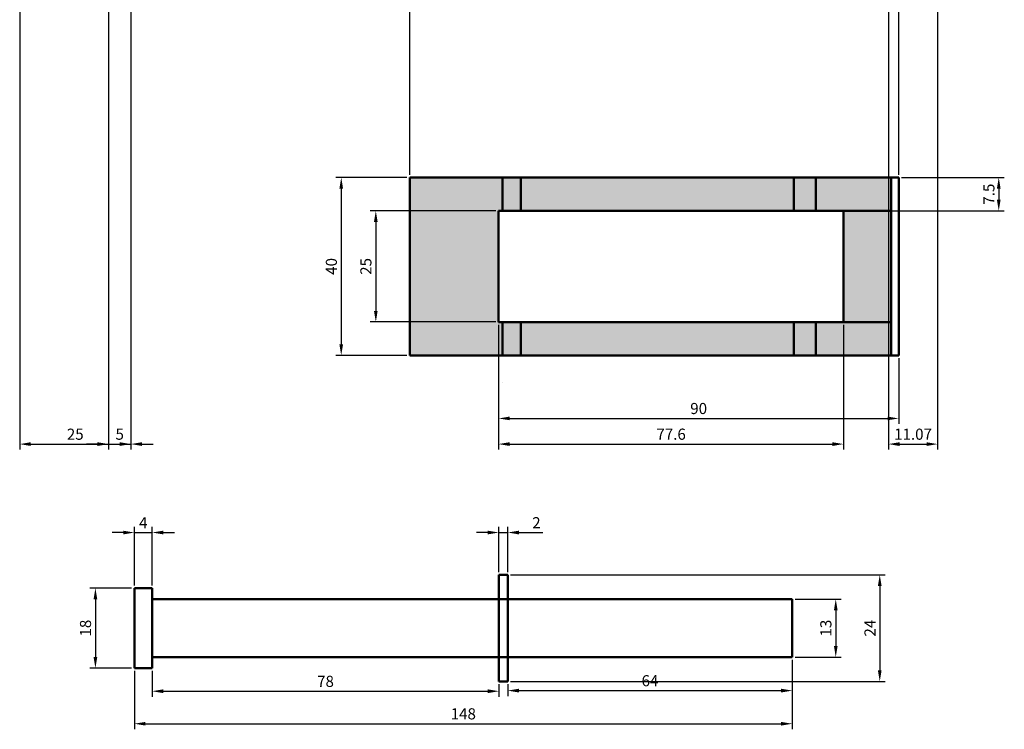
# Model space of a CAD drawing. Units: millimetres. Extents: x 2180 to 2428, y 1025 to 1371.
# Tile 1 of 3: x 2201 to 2422, y 1025 to 1185. Entities that reach past the tile are written whole.
import ezdxf

# ---------------------------------------------------------------- set-up
doc = ezdxf.new("R2010")
doc.units = ezdxf.units.MM
for name, color, linetype, lineweight in [('M-CONS', 8, 'Continuous', 13), ('M-DIMS', 2, 'Continuous', 25), ('M-HATC', 252, 'Continuous', 18), ('M-OUTL', 7, 'Continuous', 50)]:
    doc.layers.add(name, color=color, linetype=linetype, lineweight=lineweight)
doc.styles.get("Standard").update_dxf_attribs({"font": 'arial.ttf'})
doc.dimstyles.new('ISO-25', dxfattribs={"dimtxt": 2.5, "dimasz": 2.5, "dimexe": 1.25, "dimexo": 0.625, "dimtad": 1, "dimtxsty": 'Standard', "dimcen": 2.5, "dimadec": 0, "dimazin": 0, "dimtfac": 1, "dimtmove": 0, "dimatfit": 3, "dimfxl": 1, "dimarcsym": 0})

# ---------------------------------------------------------------- blocks, each defined once
blk = doc.blocks.new('*D22')
at = {"layer": 'Defpoints', "color": 0, "transparency": 16777216}
for p in [(2308.57, 1117), (2398.57, 1109.5), (2398.57, 1095.31)]:
    blk.add_point(p, dxfattribs=at)
at = {"layer": 'M-DIMS', "color": 0, "lineweight": -2, "transparency": 16777216}
for p, q in [((2308.57, 1116.37), (2308.57, 1094.06)), ((2398.57, 1108.87), (2398.57, 1094.06)), ((2311.07, 1095.31), (2396.07, 1095.31))]:
    blk.add_line(p, q, dxfattribs=at)
at = {"layer": 'M-DIMS', "color": 0, "transparency": 16777216}
for points in [[(2311.07, 1095.73), (2311.07, 1094.9), (2308.57, 1095.31)], [(2396.07, 1095.73), (2396.07, 1094.9), (2398.57, 1095.31)]]:
    blk.add_solid(points, dxfattribs=at)
at = {"layer": 'M-DIMS', "color": 0, "transparency": 16777216, "insert": (2353.57, 1097.22), "char_height": 2.5, "attachment_point": 5}
blk.add_mtext('90', dxfattribs=at)
blk = doc.blocks.new('*D23')
at = {"layer": 'Defpoints', "color": 0, "transparency": 16777216}
for p in [(2308.57, 1142), (2280.94, 1117), (2308.57, 1117)]:
    blk.add_point(p, dxfattribs=at)
at = {"layer": 'M-DIMS', "color": 0, "lineweight": -2, "transparency": 16777216}
for p, q in [((2307.95, 1142), (2279.69, 1142)), ((2280.94, 1139.5), (2280.94, 1119.5)), ((2307.95, 1117), (2279.69, 1117))]:
    blk.add_line(p, q, dxfattribs=at)
at = {"layer": 'M-DIMS', "color": 0, "transparency": 16777216}
for points in [[(2280.52, 1139.5), (2281.35, 1139.5), (2280.94, 1142)], [(2280.52, 1119.5), (2281.35, 1119.5), (2280.94, 1117)]]:
    blk.add_solid(points, dxfattribs=at)
at = {"layer": 'M-DIMS', "color": 0, "transparency": 16777216, "insert": (2279.03, 1129.5), "char_height": 2.5, "attachment_point": 5, "rotation": 90}
blk.add_mtext('25', dxfattribs=at)
blk = doc.blocks.new('*D24')
at = {"layer": 'Defpoints', "color": 0, "transparency": 16777216}
for p in [(2288.57, 1149.5), (2273.16, 1109.5), (2288.57, 1109.5)]:
    blk.add_point(p, dxfattribs=at)
at = {"layer": 'M-DIMS', "color": 0, "lineweight": -2, "transparency": 16777216}
for p, q in [((2287.95, 1149.5), (2271.91, 1149.5)), ((2273.16, 1147), (2273.16, 1112)), ((2287.95, 1109.5), (2271.91, 1109.5))]:
    blk.add_line(p, q, dxfattribs=at)
at = {"layer": 'M-DIMS', "color": 0, "transparency": 16777216}
for points in [[(2272.74, 1147), (2273.57, 1147), (2273.16, 1149.5)], [(2272.74, 1112), (2273.57, 1112), (2273.16, 1109.5)]]:
    blk.add_solid(points, dxfattribs=at)
at = {"layer": 'M-DIMS', "color": 0, "transparency": 16777216, "insert": (2271.26, 1129.5), "char_height": 2.5, "attachment_point": 5, "rotation": 90}
blk.add_mtext('40', dxfattribs=at)
blk = doc.blocks.new('*D25')
at = {"layer": 'Defpoints', "color": 0, "transparency": 16777216}
for p in [(2230.62, 1039.15), (2308.62, 1036.15), (2308.62, 1033.96)]:
    blk.add_point(p, dxfattribs=at)
at = {"layer": 'M-DIMS', "color": 0, "lineweight": -2, "transparency": 16777216}
for p, q in [((2230.62, 1038.52), (2230.62, 1032.71)), ((2308.62, 1035.52), (2308.62, 1032.71)), ((2233.12, 1033.96), (2306.12, 1033.96))]:
    blk.add_line(p, q, dxfattribs=at)
at = {"layer": 'M-DIMS', "color": 0, "transparency": 16777216}
for points in [[(2233.12, 1034.38), (2233.12, 1033.54), (2230.62, 1033.96)], [(2306.12, 1034.38), (2306.12, 1033.54), (2308.62, 1033.96)]]:
    blk.add_solid(points, dxfattribs=at)
at = {"layer": 'M-DIMS', "color": 0, "transparency": 16777216, "insert": (2269.62, 1035.86), "char_height": 2.5, "attachment_point": 5}
blk.add_mtext('78', dxfattribs=at)
blk = doc.blocks.new('*D26')
at = {"layer": 'Defpoints', "color": 0, "transparency": 16777216}
for p in [(2374.62, 1041.65), (2310.62, 1036.15), (2374.62, 1034.1)]:
    blk.add_point(p, dxfattribs=at)
at = {"layer": 'M-DIMS', "color": 0, "lineweight": -2, "transparency": 16777216}
for p, q in [((2374.62, 1041.02), (2374.62, 1032.85)), ((2310.62, 1035.52), (2310.62, 1032.85)), ((2313.12, 1034.1), (2372.12, 1034.1))]:
    blk.add_line(p, q, dxfattribs=at)
at = {"layer": 'M-DIMS', "color": 0, "transparency": 16777216}
for points in [[(2313.12, 1034.52), (2313.12, 1033.68), (2310.62, 1034.1)], [(2372.12, 1034.52), (2372.12, 1033.68), (2374.62, 1034.1)]]:
    blk.add_solid(points, dxfattribs=at)
at = {"layer": 'M-DIMS', "color": 0, "transparency": 16777216, "insert": (2342.62, 1036), "char_height": 2.5, "attachment_point": 5}
blk.add_mtext('64', dxfattribs=at)
blk = doc.blocks.new('*D27')
at = {"layer": 'Defpoints', "color": 0, "transparency": 16777216}
for p in [(2226.62, 1057.15), (2217.85, 1039.15), (2226.62, 1039.15)]:
    blk.add_point(p, dxfattribs=at)
at = {"layer": 'M-DIMS', "color": 0, "lineweight": -2, "transparency": 16777216}
for p, q in [((2226, 1057.15), (2216.6, 1057.15)), ((2217.85, 1054.65), (2217.85, 1041.65)), ((2226, 1039.15), (2216.6, 1039.15))]:
    blk.add_line(p, q, dxfattribs=at)
at = {"layer": 'M-DIMS', "color": 0, "transparency": 16777216}
for points in [[(2217.44, 1054.65), (2218.27, 1054.65), (2217.85, 1057.15)], [(2217.44, 1041.65), (2218.27, 1041.65), (2217.85, 1039.15)]]:
    blk.add_solid(points, dxfattribs=at)
at = {"layer": 'M-DIMS', "color": 0, "transparency": 16777216, "insert": (2215.95, 1048.15), "char_height": 2.5, "attachment_point": 5, "rotation": 90}
blk.add_mtext('18', dxfattribs=at)
blk = doc.blocks.new('*D28')
at = {"layer": 'Defpoints', "color": 0, "transparency": 16777216}
for p in [(2310.62, 1060.15), (2310.62, 1036.15), (2394.31, 1036.15)]:
    blk.add_point(p, dxfattribs=at)
at = {"layer": 'M-DIMS', "color": 0, "lineweight": -2, "transparency": 16777216}
for p, q in [((2311.25, 1060.15), (2395.56, 1060.15)), ((2394.31, 1057.65), (2394.31, 1038.65)), ((2311.25, 1036.15), (2395.56, 1036.15))]:
    blk.add_line(p, q, dxfattribs=at)
at = {"layer": 'M-DIMS', "color": 0, "transparency": 16777216}
for points in [[(2393.89, 1057.65), (2394.72, 1057.65), (2394.31, 1060.15)], [(2393.89, 1038.65), (2394.72, 1038.65), (2394.31, 1036.15)]]:
    blk.add_solid(points, dxfattribs=at)
at = {"layer": 'M-DIMS', "color": 0, "transparency": 16777216, "insert": (2392.43, 1048.15), "char_height": 2.5, "attachment_point": 5, "rotation": 90}
blk.add_mtext('24', dxfattribs=at)
blk = doc.blocks.new('*D29')
at = {"layer": 'Defpoints', "color": 0, "transparency": 16777216}
for p in [(2374.62, 1054.65), (2374.62, 1041.65), (2384.41, 1041.65)]:
    blk.add_point(p, dxfattribs=at)
at = {"layer": 'M-DIMS', "color": 0, "lineweight": -2, "transparency": 16777216}
for p, q in [((2375.25, 1054.65), (2385.66, 1054.65)), ((2384.41, 1052.15), (2384.41, 1044.15)), ((2375.25, 1041.65), (2385.66, 1041.65))]:
    blk.add_line(p, q, dxfattribs=at)
at = {"layer": 'M-DIMS', "color": 0, "transparency": 16777216}
for points in [[(2384, 1052.15), (2384.83, 1052.15), (2384.41, 1054.65)], [(2384, 1044.15), (2384.83, 1044.15), (2384.41, 1041.65)]]:
    blk.add_solid(points, dxfattribs=at)
at = {"layer": 'M-DIMS', "color": 0, "transparency": 16777216, "insert": (2382.51, 1048.15), "char_height": 2.5, "attachment_point": 5, "rotation": 90}
blk.add_mtext('13', dxfattribs=at)
blk = doc.blocks.new('*D30')
at = {"layer": 'Defpoints', "color": 0, "transparency": 16777216}
for p in [(2200.82, 1194.18), (2225.82, 1194.18), (2225.82, 1089.54)]:
    blk.add_point(p, dxfattribs=at)
at = {"layer": 'M-DIMS', "color": 0, "lineweight": -2, "transparency": 16777216}
for p, q in [((2200.82, 1193.55), (2200.82, 1088.29)), ((2225.82, 1193.55), (2225.82, 1088.29)), ((2203.32, 1089.54), (2223.32, 1089.54))]:
    blk.add_line(p, q, dxfattribs=at)
at = {"layer": 'M-DIMS', "color": 0, "transparency": 16777216}
for points in [[(2203.32, 1089.96), (2203.32, 1089.12), (2200.82, 1089.54)], [(2223.32, 1089.96), (2223.32, 1089.12), (2225.82, 1089.54)]]:
    blk.add_solid(points, dxfattribs=at)
at = {"layer": 'M-DIMS', "color": 0, "transparency": 16777216, "insert": (2213.32, 1091.44), "char_height": 2.5, "attachment_point": 5}
blk.add_mtext('25', dxfattribs=at)
blk = doc.blocks.new('*D34')
at = {"layer": 'Defpoints', "color": 0, "transparency": 16777216}
for p in [(2220.82, 1234.18), (2225.82, 1234.18), (2225.82, 1089.54)]:
    blk.add_point(p, dxfattribs=at)
at = {"layer": 'M-DIMS', "color": 0, "lineweight": -2, "transparency": 16777216}
for p, q in [((2220.82, 1233.55), (2220.82, 1088.29)), ((2225.82, 1233.55), (2225.82, 1088.29)), ((2218.32, 1089.54), (2215.82, 1089.54)), ((2220.82, 1089.54), (2225.82, 1089.54)), ((2228.32, 1089.54), (2230.82, 1089.54))]:
    blk.add_line(p, q, dxfattribs=at)
at = {"layer": 'M-DIMS', "color": 0, "transparency": 16777216}
for points in [[(2218.32, 1089.96), (2218.32, 1089.12), (2220.82, 1089.54)], [(2228.32, 1089.96), (2228.32, 1089.12), (2225.82, 1089.54)]]:
    blk.add_solid(points, dxfattribs=at)
at = {"layer": 'M-DIMS', "color": 0, "transparency": 16777216, "insert": (2223.32, 1091.44), "char_height": 2.5, "attachment_point": 5}
blk.add_mtext('5', dxfattribs=at)
blk = doc.blocks.new('*D37')
at = {"layer": 'Defpoints', "color": 0, "transparency": 16777216}
for p in [(2396.26, 1228.33), (2407.33, 1228.24), (2407.33, 1089.54)]:
    blk.add_point(p, dxfattribs=at)
at = {"layer": 'M-DIMS', "color": 0, "lineweight": -2, "transparency": 16777216}
for p, q in [((2396.26, 1227.71), (2396.26, 1088.29)), ((2407.33, 1227.61), (2407.33, 1088.29)), ((2398.76, 1089.54), (2404.83, 1089.54))]:
    blk.add_line(p, q, dxfattribs=at)
at = {"layer": 'M-DIMS', "color": 0, "transparency": 16777216}
for points in [[(2398.76, 1089.96), (2398.76, 1089.12), (2396.26, 1089.54)], [(2404.83, 1089.96), (2404.83, 1089.12), (2407.33, 1089.54)]]:
    blk.add_solid(points, dxfattribs=at)
at = {"layer": 'M-DIMS', "color": 0, "transparency": 16777216, "insert": (2401.8, 1091.44), "char_height": 2.5, "attachment_point": 5}
blk.add_mtext('11.07', dxfattribs=at)
blk = doc.blocks.new('*D41')
at = {"layer": 'Defpoints', "color": 0, "transparency": 16777216}
for p in [(2398.57, 1367.93), (2288.57, 1149.5), (2398.57, 1149.5)]:
    blk.add_point(p, dxfattribs=at)
at = {"layer": 'M-DIMS', "color": 0, "lineweight": -2, "transparency": 16777216}
for p, q in [((2288.57, 1150.12), (2288.57, 1369.18)), ((2398.57, 1150.12), (2398.57, 1369.18)), ((2291.07, 1367.93), (2396.07, 1367.93))]:
    blk.add_line(p, q, dxfattribs=at)
at = {"layer": 'M-DIMS', "color": 0, "transparency": 16777216}
for points in [[(2291.07, 1368.35), (2291.07, 1367.51), (2288.57, 1367.93)], [(2396.07, 1368.35), (2396.07, 1367.51), (2398.57, 1367.93)]]:
    blk.add_solid(points, dxfattribs=at)
at = {"layer": 'M-DIMS', "color": 0, "transparency": 16777216, "insert": (2343.57, 1369.83), "char_height": 2.5, "attachment_point": 5}
blk.add_mtext('110', dxfattribs=at)
blk = doc.blocks.new('*D42')
at = {"layer": 'Defpoints', "color": 0, "transparency": 16777216}
for p in [(2308.57, 1117), (2386.17, 1117), (2386.17, 1089.54)]:
    blk.add_point(p, dxfattribs=at)
at = {"layer": 'M-DIMS', "color": 0, "lineweight": -2, "transparency": 16777216}
for p, q in [((2308.57, 1116.37), (2308.57, 1088.29)), ((2386.17, 1116.37), (2386.17, 1088.29)), ((2311.07, 1089.54), (2383.67, 1089.54))]:
    blk.add_line(p, q, dxfattribs=at)
at = {"layer": 'M-DIMS', "color": 0, "transparency": 16777216}
for points in [[(2311.07, 1089.96), (2311.07, 1089.12), (2308.57, 1089.54)], [(2383.67, 1089.96), (2383.67, 1089.12), (2386.17, 1089.54)]]:
    blk.add_solid(points, dxfattribs=at)
at = {"layer": 'M-DIMS', "color": 0, "transparency": 16777216, "insert": (2347.37, 1091.44), "char_height": 2.5, "attachment_point": 5}
blk.add_mtext('77.6', dxfattribs=at)
blk = doc.blocks.new('*D43')
at = {"layer": 'Defpoints', "color": 0, "transparency": 16777216}
for p in [(2398.57, 1149.5), (2386.17, 1142), (2421.08, 1142)]:
    blk.add_point(p, dxfattribs=at)
at = {"layer": 'M-DIMS', "color": 0, "lineweight": -2, "transparency": 16777216}
for p, q in [((2399.2, 1149.5), (2422.33, 1149.5)), ((2421.08, 1147), (2421.08, 1144.5)), ((2386.8, 1142), (2422.33, 1142))]:
    blk.add_line(p, q, dxfattribs=at)
at = {"layer": 'M-DIMS', "color": 0, "transparency": 16777216}
for points in [[(2420.67, 1147), (2421.5, 1147), (2421.08, 1149.5)], [(2420.67, 1144.5), (2421.5, 1144.5), (2421.08, 1142)]]:
    blk.add_solid(points, dxfattribs=at)
at = {"layer": 'M-DIMS', "color": 0, "transparency": 16777216, "insert": (2419.19, 1145.75), "char_height": 2.5, "attachment_point": 5, "rotation": 90}
blk.add_mtext('7.5', dxfattribs=at)
blk = doc.blocks.new('*D44')
at = {"layer": 'Defpoints', "color": 0, "transparency": 16777216}
for p in [(2374.62, 1041.65), (2226.62, 1039.15), (2374.62, 1026.65)]:
    blk.add_point(p, dxfattribs=at)
at = {"layer": 'M-DIMS', "color": 0, "lineweight": -2, "transparency": 16777216}
for p, q in [((2374.62, 1041.02), (2374.62, 1025.4)), ((2226.62, 1038.52), (2226.62, 1025.4)), ((2229.12, 1026.65), (2372.12, 1026.65))]:
    blk.add_line(p, q, dxfattribs=at)
at = {"layer": 'M-DIMS', "color": 0, "transparency": 16777216}
for points in [[(2229.12, 1027.06), (2229.12, 1026.23), (2226.62, 1026.65)], [(2372.12, 1027.06), (2372.12, 1026.23), (2374.62, 1026.65)]]:
    blk.add_solid(points, dxfattribs=at)
at = {"layer": 'M-DIMS', "color": 0, "transparency": 16777216, "insert": (2300.62, 1028.55), "char_height": 2.5, "attachment_point": 5}
blk.add_mtext('148', dxfattribs=at)
blk = doc.blocks.new('*D45')
at = {"layer": 'Defpoints', "color": 0, "transparency": 16777216}
for p in [(2230.62, 1069.65), (2226.62, 1057.15), (2230.62, 1057.15)]:
    blk.add_point(p, dxfattribs=at)
at = {"layer": 'M-DIMS', "color": 0, "lineweight": -2, "transparency": 16777216}
for p, q in [((2226.62, 1057.77), (2226.62, 1070.9)), ((2230.62, 1057.77), (2230.62, 1070.9)), ((2224.12, 1069.65), (2221.62, 1069.65)), ((2226.62, 1069.65), (2230.62, 1069.65)), ((2233.12, 1069.65), (2235.62, 1069.65))]:
    blk.add_line(p, q, dxfattribs=at)
at = {"layer": 'M-DIMS', "color": 0, "transparency": 16777216}
for points in [[(2224.12, 1070.06), (2224.12, 1069.23), (2226.62, 1069.65)], [(2233.12, 1070.06), (2233.12, 1069.23), (2230.62, 1069.65)]]:
    blk.add_solid(points, dxfattribs=at)
at = {"layer": 'M-DIMS', "color": 0, "transparency": 16777216, "insert": (2228.62, 1071.52), "char_height": 2.5, "attachment_point": 5}
blk.add_mtext('4', dxfattribs=at)
blk = doc.blocks.new('*D46')
at = {"layer": 'Defpoints', "color": 0, "transparency": 16777216}
for p in [(2310.62, 1069.65), (2308.62, 1060.15), (2310.62, 1060.15)]:
    blk.add_point(p, dxfattribs=at)
at = {"layer": 'M-DIMS', "color": 0, "lineweight": -2, "transparency": 16777216}
for p, q in [((2308.62, 1060.77), (2308.62, 1070.9)), ((2310.62, 1060.77), (2310.62, 1070.9)), ((2306.12, 1069.65), (2303.62, 1069.65)), ((2308.62, 1069.65), (2310.62, 1069.65)), ((2313.12, 1069.65), (2318.53, 1069.65))]:
    blk.add_line(p, q, dxfattribs=at)
at = {"layer": 'M-DIMS', "color": 0, "transparency": 16777216}
for points in [[(2306.12, 1070.06), (2306.12, 1069.23), (2308.62, 1069.65)], [(2313.12, 1070.06), (2313.12, 1069.23), (2310.62, 1069.65)]]:
    blk.add_solid(points, dxfattribs=at)
at = {"layer": 'M-DIMS', "color": 0, "transparency": 16777216, "insert": (2317.07, 1071.53), "char_height": 2.5, "attachment_point": 5}
blk.add_mtext('2', dxfattribs=at)

msp = doc.modelspace()

# ---------------------------------------------------------------- hatches: boundary and pattern name
at = {"layer": 'M-HATC'}
h = msp.add_hatch(color=256, dxfattribs=at)
h.set_gradient(color1=(100, 33, 101), color2=(100, 33, 101), tint=1)
h.paths.add_polyline_path([(2309.4259, 1149.4968), (2288.5713, 1149.4968), (2288.5713, 1109.4968), (2309.4259, 1109.4968), (2309.4259, 1116.9968), (2308.5713, 1116.9968), (2308.5713, 1141.9968), (2309.4259, 1141.9968)])
h.paths.add_polyline_path([(2374.9543, 1149.4968), (2313.5713, 1149.4968), (2313.5713, 1141.9968), (2374.9543, 1141.9968)])
h.paths.add_polyline_path([(2313.5713, 1149.4968), (2309.4259, 1149.4968), (2309.4259, 1141.9968), (2313.5713, 1141.9968)])
h.paths.add_polyline_path([(2379.9543, 1149.4968), (2374.9543, 1149.4968), (2374.9543, 1141.9968), (2379.9543, 1141.9968)])
h.paths.add_polyline_path([(2396.8834, 1149.4968), (2379.9543, 1149.4968), (2379.9543, 1141.9968), (2396.8834, 1141.9968)])
h.paths.add_polyline_path([(2396.8834, 1141.9968), (2386.1708, 1141.9968), (2386.1708, 1116.9968), (2396.8834, 1116.9968)])
h.paths.add_polyline_path([(2396.8834, 1116.9968), (2386.1708, 1116.9968), (2379.9543, 1116.9968), (2379.9543, 1109.4968), (2396.8834, 1109.4968)])
h.paths.add_polyline_path([(2379.9543, 1116.9968), (2374.9543, 1116.9968), (2374.9543, 1109.4968), (2379.9543, 1109.4968)])
h.paths.add_polyline_path([(2374.9543, 1116.9968), (2313.5713, 1116.9968), (2313.5713, 1109.4968), (2374.9543, 1109.4968)])
h.paths.add_polyline_path([(2313.5713, 1116.9968), (2309.4259, 1116.9968), (2309.4259, 1109.4968), (2313.5713, 1109.4968)])

# ---------------------------------------------------------------- linework, layer by layer
at = {"layer": 'M-CONS'}
msp.add_line((2309.4259, 1103.2904), (2309.4259, 1103.2904), dxfattribs=at)
at = {"layer": 'M-OUTL'}
for p, q in [((2288.5713, 1149.4968), (2288.5713, 1109.4968)), ((2398.5713, 1149.4968), (2288.5713, 1149.4968)), ((2309.4259, 1149.4968), (2309.4259, 1141.9968)), ((2398.5713, 1149.4968), (2313.5713, 1149.4968)), ((2313.5713, 1149.4968), (2313.5713, 1141.9968)), ((2374.9543, 1141.9968), (2374.9543, 1149.4968)), ((2379.9543, 1149.4968), (2379.9543, 1141.9968)), ((2396.8834, 1149.4968), (2396.8834, 1109.4968)), ((2398.5713, 1109.4968), (2398.5713, 1149.4968)), ((2313.5713, 1141.9968), (2308.5713, 1141.9968)), ((2308.5713, 1141.9968), (2308.5713, 1116.9968)), ((2313.5713, 1141.9968), (2396.8834, 1141.9968)), ((2386.1708, 1141.9968), (2386.1708, 1116.9968)), ((2308.5713, 1116.9968), (2313.5713, 1116.9968)), ((2309.4259, 1116.9968), (2309.4259, 1109.4968)), ((2313.5713, 1109.4968), (2313.5713, 1116.9968)), ((2313.5713, 1116.9968), (2396.8834, 1116.9968)), ((2374.9543, 1109.4968), (2374.9543, 1116.9968)), ((2379.9543, 1116.9968), (2379.9543, 1109.4968)), ((2288.5713, 1109.4968), (2398.5713, 1109.4968)), ((2398.5713, 1109.4968), (2313.5713, 1109.4968)), ((2308.6201, 1048.1463), (2308.6201, 1060.1463)), ((2308.6201, 1060.1463), (2310.6201, 1060.1463)), ((2310.6201, 1060.1463), (2310.6201, 1036.1463)), ((2226.6201, 1057.1463), (2226.6201, 1039.1463)), ((2230.6201, 1057.1463), (2226.6201, 1057.1463)), ((2230.6201, 1039.1463), (2230.6201, 1057.1463)), ((2230.6201, 1057.1463), (2230.6201, 1054.6463)), ((2310.6201, 1054.6463), (2310.6201, 1057.6463)), ((2230.6201, 1054.6463), (2374.6201, 1054.6463)), ((2310.6201, 1041.6463), (2310.6201, 1054.6463)), ((2374.6201, 1041.6463), (2374.6201, 1054.6463)), ((2308.6201, 1036.1463), (2308.6201, 1048.1463)), ((2230.6201, 1039.1463), (2230.6201, 1041.6463)), ((2230.6201, 1041.6463), (2374.6201, 1041.6463)), ((2374.6201, 1041.6463), (2310.6201, 1041.6463)), ((2226.6201, 1039.1463), (2230.6201, 1039.1463)), ((2310.6201, 1036.1463), (2308.6201, 1036.1463))]:
    msp.add_line(p, q, dxfattribs=at)

# ---------------------------------------------------------------- dimensions: what is measured, and where the dimension line sits
at = {"layer": 'M-DIMS'}
for base, p1, p2, override, picture, middle in [((2398.5713, 1367.9295), (2288.5713, 1149.4968), (2398.5713, 1149.4968), {"dimdec": 0, "dimlfac": 1, "dimrnd": 0, "dimzin": 0, "dimdsep": 46, "dimlunit": 2}, '*D41', (2343.5713, 1369.831)), ((2225.8192, 1089.5404), (2220.8192, 1234.1795), (2225.8192, 1234.1795), {"dimdec": 0, "dimlfac": 1, "dimrnd": 0, "dimzin": 0, "dimdsep": 46, "dimlunit": 2}, '*D34', (2223.3192, 1091.4367)), ((2407.3324, 1089.5404), (2396.2634, 1228.3311), (2407.3324, 1228.2381), {"dimdec": 2, "dimlfac": 1, "dimrnd": 0, "dimzin": 0, "dimdsep": 46, "dimlunit": 2}, '*D37', (2401.7979, 1091.4418)), ((2225.8192, 1089.5404), (2200.8192, 1194.1795), (2225.8192, 1194.1795), {"dimdec": 0, "dimlfac": 1, "dimrnd": 0, "dimzin": 0, "dimdsep": 46, "dimlunit": 2}, '*D30', (2213.3192, 1091.4418)), ((2398.5713, 1095.3141), (2308.5713, 1116.9968), (2398.5713, 1109.4968), {"dimclrd": 0, "dimclre": 0, "dimclrt": 0}, '*D22', (2353.5713, 1097.2155)), ((2386.1708, 1089.5404), (2308.5713, 1116.9968), (2386.1708, 1116.9968), {"dimdec": 1, "dimlfac": 1, "dimrnd": 0, "dimzin": 0, "dimdsep": 46, "dimlunit": 2}, '*D42', (2347.3711, 1091.4418)), ((2230.6201, 1069.6463), (2226.6201, 1057.1463), (2230.6201, 1057.1463), {"dimdec": 0, "dimlfac": 1, "dimrnd": 0, "dimzin": 0, "dimdsep": 46, "dimlunit": 2}, '*D45', (2228.6201, 1071.5213)), ((2310.6201, 1069.6463), (2308.6201, 1060.1463), (2310.6201, 1060.1463), {"dimdec": 0, "dimlfac": 1, "dimrnd": 0, "dimzin": 0, "dimdsep": 46, "dimlunit": 2}, '*D46', (2317.0731, 1071.5265)), ((2374.6201, 1026.6463), (2226.6201, 1039.1463), (2374.6201, 1041.6463), {"dimdec": 0, "dimlfac": 1, "dimrnd": 0, "dimzin": 0, "dimdsep": 46, "dimlunit": 2}, '*D44', (2300.6201, 1028.5478)), ((2374.6201, 1034.0986), (2310.6201, 1036.1463), (2374.6201, 1041.6463), {"dimclrd": 0, "dimclre": 0, "dimclrt": 0}, '*D26', (2342.6201, 1036)), ((2308.6201, 1033.9613), (2230.6201, 1039.1463), (2308.6201, 1036.1463), {"dimclrd": 0, "dimclre": 0, "dimclrt": 0}, '*D25', (2269.6201, 1035.8627))]:
    dim = msp.add_linear_dim(base=base, p1=p1, p2=p2, dimstyle='ISO-25', override=override, dxfattribs=at)
    dim.commit()
    dim.dimension.update_dxf_attribs({"geometry": picture, "text_midpoint": middle})
for base, p1, p2, override, picture, middle in [((2273.1578, 1109.4968), (2288.5713, 1149.4968), (2288.5713, 1109.4968), {"dimclrd": 0, "dimclre": 0, "dimclrt": 0}, '*D24', (2271.2564, 1129.4968)), ((2421.0824, 1141.9968), (2398.5713, 1149.4968), (2386.1708, 1141.9968), {"dimdec": 1, "dimlfac": 1, "dimrnd": 0, "dimzin": 0, "dimdsep": 46, "dimlunit": 2}, '*D43', (2419.1861, 1145.7468)), ((2280.9363, 1116.9968), (2308.5713, 1141.9968), (2308.5713, 1116.9968), {"dimclrd": 0, "dimclre": 0, "dimclrt": 0}, '*D23', (2279.0348, 1129.4968)), ((2394.3063, 1036.1463), (2310.6201, 1060.1463), (2310.6201, 1036.1463), {"dimclrd": 0, "dimclre": 0, "dimclrt": 0}, '*D28', (2392.4262, 1048.1463)), ((2217.8535, 1039.1463), (2226.6201, 1057.1463), (2226.6201, 1039.1463), {"dimclrd": 0, "dimclre": 0, "dimclrt": 0}, '*D27', (2215.952, 1048.1463)), ((2384.4118, 1041.6463), (2374.6201, 1054.6463), (2374.6201, 1041.6463), {"dimclrd": 0, "dimclre": 0, "dimclrt": 0}, '*D29', (2382.5095, 1048.1463))]:
    dim = msp.add_linear_dim(base=base, p1=p1, p2=p2, angle=90, dimstyle='ISO-25', override=override, dxfattribs=at)
    dim.commit()
    dim.dimension.update_dxf_attribs({"geometry": picture, "text_midpoint": middle})

doc.saveas('drawing.dxf')
